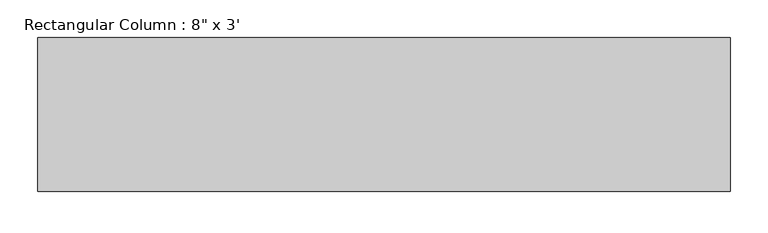
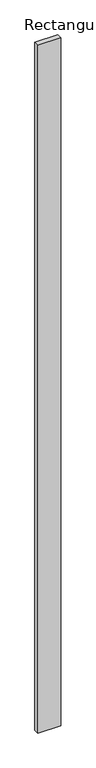
"""IFC4 building model written with IfcOpenShell, lengths in millimetres: column geometry."""

from ifc_helpers import new_model, si_unit, origin, origin_with_axes, place, context, project, spatial, polyline, outline, extrude, source, transform, mapped, element, save


def column_7936e864(model_context):
    return source(origin(), model_context, "Body", "SweptSolid", [
        extrude(outline(polyline([(457.2, 101.6), (457.2, -101.6), (-457.2, -101.6), (-457.2, 101.6), (457.2, 101.6)])), origin_with_axes(), (0.0, 0.0, 1.0), 29108.4),
    ])


if __name__ == "__main__":
    model = new_model("IFC4")
    model_context = context("Model", 3, world=origin())
    ifc_project = project(units=[si_unit("LENGTHUNIT", "METRE", prefix="MILLI")], contexts=[model_context])
    site = spatial("IfcSite", under=ifc_project)
    building = spatial("IfcBuilding", under=site)
    placement = place(None, origin())
    column_shape = column_7936e864(model_context)
    element("IfcColumn", 1, ObjectType="Rectangular Column : 8\" x 3'", at=placement, inside=building, context=model_context, shape_type="MappedRepresentation", body=[
        mapped(column_shape, transform((0.0, 0.0, 0.0), x_axis=(1.0, 0.0, 0.0), y_axis=(0.0, 1.0, 0.0), z_axis=(0.0, 0.0, 1.0))),
    ])
    save(model, "model.ifc")

# Revit data of these elements
# Type "Rectangular Column : 8\" x 3'"
#   Assembly Code = "B1010200"
#   Depth = 0' - 8"
#   Offset Base = 0' - 0"
#   Offset Top = 0' - 0"
#   Width = 3' - 0"
#   Material = none
